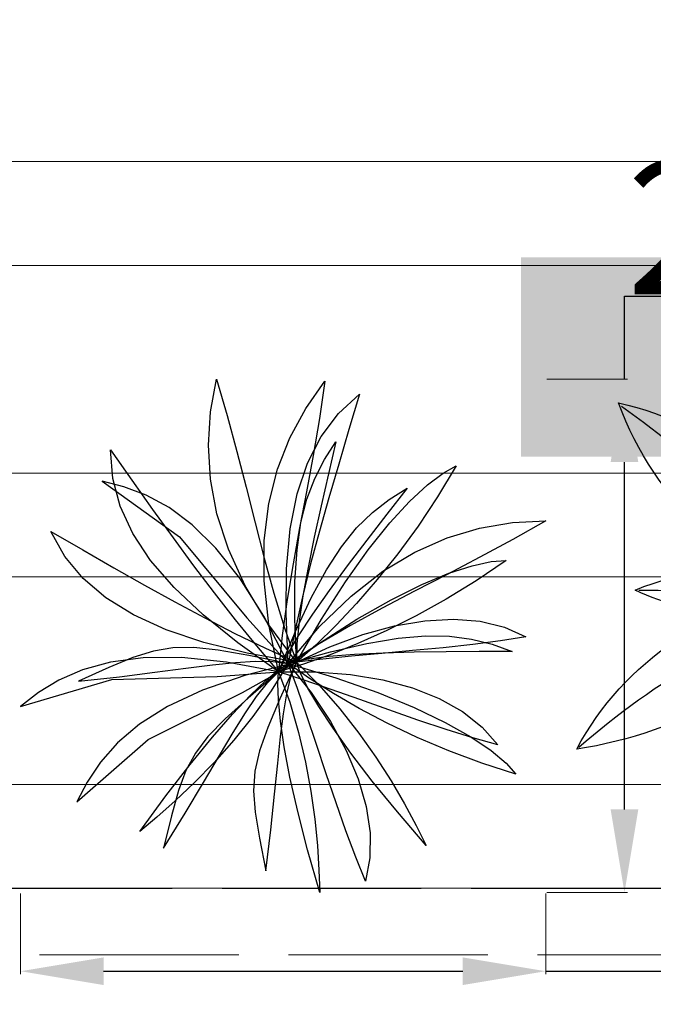
# Model space of a CAD drawing. Units: inches. Extents: x 351 to 1738, y -265 to 286.
# Tile 10 of 38: x 1074 to 1112, y -206 to -147. Entities that reach past the tile are written whole.
import ezdxf

# ---------------------------------------------------------------- set-up
doc = ezdxf.new("R2010")
doc.units = ezdxf.units.IN
doc.header["$MEASUREMENT"] = 0
doc.linetypes.add('ACAD_ISO02W100', pattern=[15, 12, -3])
for name, color, linetype, lineweight in [('A-ANNO-DIMS', 2, 'Continuous', 18), ('A-COLS-PATT', 6, 'Continuous', 13), ('A-FLOR-OVHD', 1, 'ACAD_ISO02W100', 18), ('A-FLOR-PATT', 9, 'Continuous', 9)]:
    doc.layers.add(name, color=color, linetype=linetype, lineweight=lineweight)
for name, color, linetype in [('CAY', 94, 'Continuous'), ('CHITIET', 144, 'Continuous'), ('DIENHOA', 3, 'Continuous'), ('netmanh', 9, 'Continuous'), ('VATDUNG', 9, 'Continuous')]:
    doc.layers.add(name, color=color, linetype=linetype)
doc.styles.get("Standard").update_dxf_attribs({"font": 'arial.ttf'})
doc.dimstyles.get("Standard").update_dxf_attribs({"dimtxt": 8, "dimasz": 5, "dimexe": 0.18, "dimexo": 0.0625, "dimgap": 0.09, "dimtad": 1, "dimtoh": 1, "dimzin": 0, "dimdsep": 46, "dimlunit": 4, "dimtxsty": 'Standard', "dimcen": 0, "dimclre": 256, "dimadec": 0, "dimazin": 0, "dimtfac": 1, "dimtofl": 0, "dimtmove": 0, "dimatfit": 3, "dimfxl": 1, "dimtolj": 1, "dimtzin": 0, "dimlwe": -1, "dimarcsym": 0})

# ---------------------------------------------------------------- blocks, each defined once
blk = doc.blocks.new('Cay03_mb')
at = {"layer": 'DIENHOA'}
for p, q in [((118.6, 555.3), (166.2, 599.1)), ((166.2, 599.1), (142.2, 519.4)), ((79.5, 503.7), (118.6, 555.3)), ((142.2, 519.4), (119, 441.7)), ((48.6, 443.6), (79.5, 503.7)), ((25.5, 374.3), (48.6, 443.6)), ((119, 441.7), (96.7, 365.6)), ((-365.2, 390.3), (-414.4, 402.8)), ((-414.4, 402.8), (-240.2, 277.8)), ((-314.9, 371.3), (-365.2, 390.3)), ((-263.5, 343.5), (-314.9, 371.3)), ((9.9, 295.3), (25.5, 374.3)), ((96.7, 365.6), (75.6, 290.6)), ((-211.2, 304.6), (-263.5, 343.5)), ((511, 309.6), (585.9, 313.5)), ((585.9, 313.5), (511.8, 271.4)), ((-158, 252.3), (-211.2, 304.6)), ((1.6, 205.7), (9.9, 295.3)), ((75.6, 290.6), (55.7, 216.3)), ((363.4, 275.4), (436.8, 297.2)), ((436.8, 297.2), (511, 309.6)), ((-240.2, 277.8), (-88.4, 94.9)), ((290.6, 243.2), (363.4, 275.4)), ((511.8, 271.4), (437.6, 231.5)), ((-104.2, 184.4), (-158, 252.3)), ((218.5, 199.8), (290.6, 243.2)), ((437.6, 231.5), (363.7, 192.9)), ((0.2, 104.9), (1.6, 205.7)), ((55.7, 216.3), (37.3, 142.1)), ((-49.6, 98.5), (-104.2, 184.4)), ((147, 144.1), (218.5, 199.8)), ((363.7, 192.9), (290.2, 154.9)), ((37.3, 142.1), (20.5, 67.6)), ((75.9, 75.2), (147, 144.1)), ((290.2, 154.9), (217.4, 116.6)), ((217.4, 116.6), (145.5, 77.3)), ((-88.4, 94.9), (5.4, -7.8)), ((5.4, -7.8), (-49.6, 98.5)), ((5.4, -7.8), (0.2, 104.9)), ((5.4, -7.8), (75.9, 75.2)), ((20.5, 67.6), (5.4, -7.8)), ((145.5, 77.3), (74.7, 36.1)), ((182.2, 37.2), (253, 48.9)), ((253, 48.9), (314.6, 54.1)), ((314.6, 54.1), (369.2, 53.3)), ((369.2, 53.3), (418.6, 46.8)), ((418.6, 46.8), (464.9, 35.2)), ((-254.7, 27.4), (-298.6, 20.1)), ((-208, 27.8), (-254.7, 27.4)), ((-152.7, 21.7), (-208, 27.8)), ((74.7, 36.1), (5.4, -7.8)), ((100.3, 18.4), (182.2, 37.2)), ((464.9, 35.2), (510, 19)), ((-345, 5.4), (-399.6, -17.1)), ((-298.6, 20.1), (-345, 5.4)), ((-83.4, 9.7), (-152.7, 21.7)), ((5.4, -7.8), (-83.4, 9.7)), ((5.4, -7.8), (100.3, 18.4)), ((46.3, 0.9), (5.4, -7.8)), ((96.7, 7.5), (46.3, 0.9)), ((155, 12.2), (96.7, 7.5)), ((219.6, 15.4), (155, 12.2)), ((289, 17.4), (219.6, 15.4)), ((361.6, 18.5), (289, 17.4)), ((435.8, 18.9), (361.6, 18.5)), ((510, 19), (435.8, 18.9)), ((-399.6, -17.1), (-468, -47.9)), ((-295.3, -27.9), (-225.8, -18.9)), ((-225.8, -18.9), (-165.8, -11.3)), ((-165.8, -11.3), (-114, -5.7)), ((-114, -5.7), (-69, -2.9)), ((-69, -2.9), (-29.6, -3.4)), ((5.4, -7.8), (-33.2, -69.5)), ((-29.6, -3.4), (5.4, -7.8)), ((-16.5, -22.4), (5.4, -7.8)), ((5.4, -7.8), (56.8, -73.3)), ((25.9, -64.4), (5.4, -7.8)), ((5.4, -7.8), (112.8, -40.3)), ((53.5, -41.6), (5.4, -7.8)), ((-468, -47.9), (-375.6, -37.8)), ((-375.6, -37.8), (-295.3, -27.9)), ((-45.1, -46.3), (-16.5, -22.4)), ((107, -75.7), (53.5, -41.6)), ((112.8, -40.3), (207.5, -73.8)), ((-79.8, -79.6), (-45.1, -46.3)), ((47, -125.9), (25.9, -64.4)), ((-120.2, -122.1), (-79.8, -79.6)), ((-33.2, -69.5), (-74.6, -127.3)), ((56.8, -73.3), (100.4, -139.1)), ((165.5, -109.6), (107, -75.7)), ((207.5, -73.8), (289.5, -107.6)), ((228.7, -142.8), (165.5, -109.6)), ((289.5, -107.6), (359.3, -141.1)), ((-165.9, -174.1), (-120.2, -122.1)), ((-74.6, -127.3), (-117.8, -181.1)), ((68.7, -190.6), (47, -125.9)), ((100.4, -139.1), (135.9, -204.3)), ((296, -174.7), (228.7, -142.8)), ((359.3, -141.1), (416.9, -173.5)), ((-216.3, -235.6), (-165.9, -174.1)), ((367.1, -204.8), (296, -174.7)), ((416.9, -173.5), (462.6, -204.2)), ((-117.8, -181.1), (-162.1, -230.9)), ((90.8, -256.6), (68.7, -190.6)), ((135.9, -204.3), (162.8, -268.3)), ((441.6, -232.7), (367.1, -204.8)), ((462.6, -204.2), (496.5, -232.5)), ((-271, -306.6), (-216.3, -235.6)), ((-162.1, -230.9), (-206.3, -276.5)), ((518.9, -257.7), (441.6, -232.7)), ((496.5, -232.5), (518.9, -257.7)), ((113.1, -322.2), (90.8, -256.6)), ((-206.3, -276.5), (-249.6, -317.8)), ((162.8, -268.3), (181, -330.4)), ((-329.5, -387.1), (-271, -306.6)), ((-249.6, -317.8), (-291, -354.7)), ((135.4, -385.6), (113.1, -322.2)), ((181, -330.4), (190, -390)), ((-291, -354.7), (-329.5, -387.1)), ((157.6, -445), (135.4, -385.6)), ((190, -390), (189.6, -446.3)), ((179.5, -498.7), (157.6, -445)), ((189.6, -446.3), (179.5, -498.7))]:
    blk.add_line(p, q, dxfattribs=at)
for points in [[(23.7, -5.4), (-41, 82.2), (-91.8, 167.1), (-129.7, 249.5), (-155.6, 329.6), (-170.2, 407.8), (-174.7, 484.2), (-169.8, 559.3), (-156.5, 633.1)], [(-156.5, 633.1), (-132.5, 551.3), (-110.5, 470), (-89.8, 389.2), (-69.6, 309), (-49, 229.4), (-27.1, 150.4), (-3.2, 72.1), (23.7, -5.4)], [(-16.4, -26.7), (-38.3, 80), (-48.9, 178.3), (-48.7, 269), (-38.5, 352.6), (-19.1, 429.7), (9, 501), (44.9, 567.1), (87.9, 628.5)], [(87.9, 628.5), (75.5, 544.2), (61.3, 461.2), (46.1, 379.1), (30.8, 297.8), (16.1, 216.9), (2.9, 136), (-8.3, 54.9), (-16.4, -26.7)], [(23.7, -5.4), (19.8, 93), (20.3, 177), (25, 248.5), (34, 309.8), (47.3, 362.7), (64.9, 409.3), (86.8, 451.7), (112.9, 491.9)], [(112.9, 491.9), (96, 419.7), (79.5, 347.4), (63.9, 276.5), (50, 208.4), (38.4, 144.8), (29.7, 86.9), (24.6, 36.3), (23.7, -5.4)], [(-395.6, 473.7), (-347.5, 405.6), (-300.6, 339.5), (-254.3, 275.1), (-208.3, 212.3), (-161.9, 150.9), (-114.8, 90.7), (-66.5, 31.6), (-16.4, -26.7)], [(-16.4, -26.7), (-108.3, 38.6), (-186.9, 101.7), (-252.4, 163.5), (-305.1, 224.4), (-345.4, 285.2), (-373.7, 346.6), (-390.4, 409.2), (-395.6, 473.7)], [(384.3, 437.5), (342.2, 367.8), (298.1, 301.7), (252.6, 239.4), (206.1, 181.1), (159.4, 127.2), (113, 78), (67.6, 33.6), (23.7, -5.4)], [(23.7, -5.4), (79.9, 91.7), (134.1, 176.2), (185.8, 248.4), (234.3, 308.7), (279, 357.3), (319.3, 394.8), (354.6, 421.4), (384.3, 437.5)], [(273.2, 387.3), (227.6, 328.8), (182.3, 270.1), (138.4, 212.3), (97.2, 156.4), (60, 103.4), (27.8, 54.6), (1.9, 10.8), (-16.4, -26.7)], [(-16.4, -26.7), (21.4, 64.2), (57, 140.3), (91.4, 203.3), (125.2, 255.1), (159.5, 297.5), (195, 332.5), (232.7, 361.8), (273.2, 387.3)], [(-530.5, 289.7), (-458.3, 248.1), (-387.9, 207.8), (-318.9, 168.7), (-250.8, 131.1), (-182.9, 94.8), (-114.9, 59.9), (-46.2, 26.5), (23.7, -5.4)], [(23.7, -5.4), (-87.2, 15.2), (-185, 39.6), (-270.3, 68.2), (-343.7, 101.4), (-405.9, 139.7), (-457.3, 183.5), (-498.7, 233.4), (-530.5, 289.7)], [(496.7, 224), (429.4, 178.4), (361.6, 136.9), (294.1, 99.5), (227.5, 66.1), (162.4, 36.7), (99.7, 11.5), (39.8, -9.7), (-16.4, -26.7)], [(-16.4, -26.7), (75.4, 37.9), (160.1, 91.8), (237.3, 135.7), (306.6, 170), (367.6, 195.4), (419.9, 212.5), (463.1, 221.9), (496.7, 224)], [(23.7, -5.4), (99.3, 29.7), (173.2, 57.1), (244.8, 76.7), (313.3, 88.3), (377.9, 91.8), (437.9, 87), (492.7, 73.8), (541.4, 52)], [(541.4, 52), (484.1, 42.9), (421.2, 34.8), (354.4, 27.6), (285.4, 20.9), (216.1, 14.5), (148.2, 8.1), (83.5, 1.6), (23.7, -5.4)], [(-16.4, -26.7), (-134, -4.7), (-235.3, 5.3), (-322, 4.7), (-395.9, -5), (-458.7, -22.3), (-512.3, -45.7), (-558.2, -73.6), (-598.4, -104.7)], [(-471.9, -320.3), (-310.5, -179.3), (-97.7, -73.3), (23.7, -5.4)], [(23.7, -5.4), (-92.3, -34.8), (-188.4, -68.2), (-266.9, -105.1), (-329.9, -144.9), (-379.7, -187), (-418.5, -230.7), (-448.5, -275.3), (-471.9, -320.3)], [(23.7, -5.4), (-13.6, -87.9), (-41.1, -152.6), (-59.6, -205), (-69.9, -250.7), (-72.8, -295), (-69.2, -343.6), (-59.7, -401.9), (-45.3, -475.5)], [(-45.3, -475.5), (-34.1, -383.2), (-25.4, -302.8), (-18.3, -233.1), (-12, -172.9), (-5.6, -121.2), (2, -76.8), (11.4, -38.5), (23.7, -5.4)], [(316.5, -418.1), (251.4, -342.8), (194.8, -273.3), (146.5, -210.2), (106.3, -153.8), (74.1, -104.7), (49.7, -63.4), (32.9, -30.1), (23.7, -5.4)], [(23.7, -5.4), (74.9, -57.1), (121.8, -110.6), (164.3, -165), (202.7, -219.4), (237, -272.9), (267.3, -324.5), (293.7, -373.2), (316.5, -418.1)], [(-598.4, -104.7), (-392.7, -44.4), (-155, -37.4), (-16.4, -26.7)], [(-276.2, -424.4), (-227.3, -345.4), (-185.7, -276.1), (-150, -215.7), (-119.1, -163.8), (-91.5, -119.5), (-66, -82.3), (-41.4, -51.6), (-16.4, -26.7)], [(-16.4, -26.7), (-84.9, -86), (-137, -133.1), (-175.8, -173), (-204.3, -210), (-225.5, -249.1), (-242.5, -294.7), (-258.4, -351.6), (-276.2, -424.4)], [(76.2, -524.2), (48.8, -428.5), (26.6, -341.7), (9.2, -264.1), (-3.6, -196.1), (-12.3, -138), (-17.1, -90.2), (-18.3, -53), (-16.4, -26.7)], [(-16.4, -26.7), (66.9, -26.6), (145.6, -32.7), (218.8, -44.9), (285.8, -63.1), (345.9, -87.1), (398.4, -116.6), (442.6, -151.6), (477.6, -191.8)], [(477.6, -191.8), (421.8, -176), (361.3, -156.9), (297.6, -135.5), (232.2, -112.6), (166.6, -89.4), (102.3, -66.6), (40.8, -45.4), (-16.4, -26.7)], [(-16.4, -26.7), (8.5, -95.1), (28.5, -163.3), (44.3, -230.6), (56.3, -296.1), (65, -359), (70.9, -418.5), (74.5, -473.9), (76.2, -524.2)]]:
    blk.add_lwpolyline(points, dxfattribs=at)
blk = doc.blocks.new('A$C5431134F')
at = {"layer": 'VATDUNG'}
for centre, radius, start, end in [((2160.8, 1662), 1245, 150.2411, 205.809), ((5177, 1582.5), 4150.3, 170.24, 186.1148), ((-65.9, 1738.8), 1267.2, 354.3326, 25.2804), ((1532.8, 1250.1), 499, 101.4267, 190.9877), ((193.1, 3473.3), 2507.8, 289.6318, 316.9416), ((2357.8, 162.2), 1629.1, 101.2486, 143.9899), ((1828.1, 1082.8), 773.2, 121.9055, 175.1859), ((1000.7, 2213.1), 1133.8, 274.4073, 336.4431), ((3715.1, 660.2), 2523.5, 154.6853, 162.4501), ((-246.7, 51.1), 1647.5, 39.15, 81.389), ((1000.7, 2213.1), 1133.8, 208.0484, 264.6491), ((1859.5, 3770.4), 2797.6, 228.5745, 252.3842), ((1101.5, 1552.5), 361.2, 169.1166, 218.9556), ((667.9, 1279.8), 349.9, 42.8374, 76.9786), ((-929.9, 388.9), 2082.1, 20.5138, 36.0242), ((1386.4, 1856.4), 738.5, 261.6389, 315.6255), ((-169.9, 6392.7), 5465.7, 286.3355, 292.415), ((1571.2, 1428.8), 356.3, 257.3557, 344.3532), ((624.5, 223.6), 940.4, 92.4374, 115.2956), ((-65.9, 1738.8), 1267.2, 330.7697, 331.9367), ((1294.4, -49.6), 1206.1, 104.1284, 160.1468), ((-2233.8, 3749.8), 4146.2, 305.4464, 320.7382), ((248.9, 8461.8), 7388, 269.91003, 274.50199), ((2052.7, 864.5), 1083.3, 166.3603, 232.9474), ((1250.8, 281.5), 836.9, 19.4342, 107.4357), ((625, 349.3), 851.8, 6.5073, 62.3609), ((754.1, -691.9), 1814.1, 46.1483, 80.3711), ((-70, 1420), 1084.7, 282.2423, 341.7321), ((546.4, 1826.6), 819.5, 246.7315, 287.3971), ((3885.3, 1488.7), 2894, 188.0959, 210.7226), ((1889.6, 1210.8), 871.9, 188.5552, 241.3289), ((-527.8, -458.7), 2192.5, 24.7599, 44.6473), ((2594.9, 3037.7), 2500, 231.5416, 257.1764), ((1738.9, 617.5), 897.6, 155.9893, 202.84), ((2946.5, 414), 2039.9, 165.0604, 184.0737), ((1214.1, 597.8), 452.1, 154.5276, 228.0163), ((-246.7, 51.1), 1647.5, 358.2222, 17.8583)]:
    blk.add_arc(centre, radius, start, end, dxfattribs=at)
blk = doc.blocks.new('A$C5A8625A6')
at = {"layer": 'CHITIET', "ltscale": 50, "xscale": -0.49, "yscale": 0.49, "zscale": 0.49, "rotation": 180}
blk.add_blockref('A$C5431134F', (0, 1120.2), dxfattribs=at)
blk = doc.blocks.new('A$C18571848')
at = {"layer": 'netmanh', "xscale": 0.5393606399999998, "yscale": 0.5393606399999998, "zscale": 0.5393606399999998}
blk.add_blockref('A$C5A8625A6', (0, 0), dxfattribs=at)
blk = doc.blocks.new('*D36')
at = {"layer": 'A-ANNO-DIMS', "transparency": 16777216}
for p, q in [((1073.569, -199.341), (1073.569, -204.202)), ((1105.198, -199.341), (1105.198, -204.202))]:
    blk.add_line(p, q, dxfattribs=at)
at = {"layer": 'A-ANNO-DIMS', "color": 0, "lineweight": -2, "transparency": 16777216}
for p, q in [((1078.569, -204.022), (1100.198, -204.022)), ((1105.198, -204.022), (1227.071, -204.022))]:
    blk.add_line(p, q, dxfattribs=at)
at = {"layer": 'A-ANNO-DIMS', "color": 0, "transparency": 16777216}
for points in [[(1078.569, -203.189), (1078.569, -204.856), (1073.569, -204.022)], [(1100.198, -203.189), (1100.198, -204.856), (1105.198, -204.022)]]:
    blk.add_solid(points, dxfattribs=at)
at = {"layer": 'Defpoints', "color": 0, "transparency": 16777216}
for p in [(1073.569, -199.278), (1105.198, -199.278), (1105.198, -204.022)]:
    blk.add_point(p, dxfattribs=at)
at = {"layer": 'A-ANNO-DIMS', "color": 0, "transparency": 16777216, "insert": (1168.634, -199.796), "char_height": 8, "attachment_point": 5}
blk.add_mtext('\\A1;PLANT A 2\'-7 1/2" TYP.', dxfattribs=at)
blk = doc.blocks.new('*D37')
at = {"layer": 'A-ANNO-DIMS', "color": 0, "lineweight": -2, "transparency": 16777216}
for p, q in [((1109.942, -168.369), (1109.942, -163.369)), ((1109.942, -163.369), (1158.933, -163.369)), ((1109.942, -194.278), (1109.942, -173.369))]:
    blk.add_line(p, q, dxfattribs=at)
at = {"layer": 'A-ANNO-DIMS', "transparency": 16777216}
for p, q in [((1105.26, -168.369), (1110.122, -168.369)), ((1105.26, -199.278), (1110.122, -199.278))]:
    blk.add_line(p, q, dxfattribs=at)
at = {"layer": 'A-ANNO-DIMS', "color": 0, "transparency": 16777216}
for points in [[(1109.109, -173.369), (1110.775, -173.369), (1109.942, -168.369)], [(1109.109, -194.278), (1110.775, -194.278), (1109.942, -199.278)]]:
    blk.add_solid(points, dxfattribs=at)
at = {"layer": 'Defpoints', "color": 0, "transparency": 16777216}
for p in [(1105.198, -168.369), (1109.942, -168.369), (1105.198, -199.278)]:
    blk.add_point(p, dxfattribs=at)
at = {"layer": 'A-ANNO-DIMS', "color": 0, "transparency": 16777216, "insert": (1134.482, -159.26), "char_height": 8, "attachment_point": 5}
blk.add_mtext('\\A1;2\'-7" TYP.', dxfattribs=at)

msp = doc.modelspace()

# ---------------------------------------------------------------- hatches: boundary and pattern name
at = {"layer": 'A-COLS-PATT'}
h = msp.add_hatch(color=256, dxfattribs=at)
h.dxf.hatch_style = 1
h.paths.add_polyline_path([(1112.704, 237.963), (1103.704, 237.963), (1103.704, 228.963), (1112.704, 228.963)])
h.paths.add_polyline_path([(1115.704, 237.963), (1112.704, 237.963), (1112.704, 228.963), (1115.704, 228.963)])
h.paths.add_polyline_path([(1043.704, 255.963), (1034.704, 255.963), (1034.704, 243.963), (1043.704, 243.963)])
h.paths.add_polyline_path([(1043.704, 210.963), (1034.704, 210.963), (1034.704, 198.963), (1043.704, 198.963)])
h.paths.add_polyline_path([(1043.704, -45.037), (1034.704, -45.037), (1034.704, -57.037), (1043.704, -57.037)])
h.paths.add_polyline_path([(1112.704, -45.037), (1103.704, -45.037), (1103.704, -57.037), (1112.704, -57.037)])
h.paths.add_polyline_path([(1112.704, -161.037), (1103.704, -161.037), (1103.704, -164.037), (1103.704, -173.037), (1112.704, -173.037)])
h.paths.add_polyline_path([(1043.704, -161.037), (1034.704, -161.037), (1034.704, -173.037), (1043.704, -173.037)])
h.paths.add_polyline_path([(1248.549, -164.037), (1236.549, -164.037), (1236.549, -173.037), (1248.549, -173.037)])
h.paths.add_polyline_path([(1248.549, -50), (1236.549, -50), (1236.549, -59), (1248.549, -59)])
h.paths.add_polyline_path([(1248.704, 73.463), (1244.704, 73.463), (1244.704, 64.463), (1248.704, 64.463)])
h.paths.add_polyline_path([(1244.704, 73.463), (1236.704, 73.463), (1236.704, 64.463), (1244.704, 64.463)])
h.paths.add_polyline_path([(1248.704, 237.963), (1236.704, 237.963), (1236.704, 228.963), (1248.704, 228.963)])
h.paths.add_polyline_path([(1392.204, 237.963), (1380.204, 237.963), (1380.204, 228.963), (1392.204, 228.963)])
h.paths.add_polyline_path([(1536.064, 237.963), (1524.064, 237.963), (1524.064, 228.963), (1536.064, 228.963)])
h.paths.add_polyline_path([(1536.064, 73.463), (1524.064, 73.463), (1524.064, 64.463), (1536.064, 64.463)])
h.paths.add_polyline_path([(1384.204, 73.463), (1380.204, 73.463), (1380.204, 64.463), (1384.204, 64.463)])
h.paths.add_polyline_path([(1392.064, 73.463), (1384.204, 73.463), (1384.204, 64.463), (1392.064, 64.463)])
h.paths.add_polyline_path([(1536.064, -53.037), (1524.064, -53.037), (1524.064, -57.037), (1536.064, -57.037)])
h.paths.add_polyline_path([(1536.064, -48.037), (1524.064, -48.037), (1524.064, -53.037), (1536.064, -53.037)])
h.paths.add_polyline_path([(1392.064, -48.037), (1380.064, -48.037), (1380.064, -56.5), (1380.065, -57.037), (1392.064, -57.037)])
h.paths.add_polyline_path([(1536.064, -164.037), (1524.064, -164.037), (1524.064, -173.037), (1536.064, -173.037)])
at = {"layer": 'A-FLOR-PATT', "transparency": 33554559}
h = msp.add_hatch(dxfattribs=at)
h.set_pattern_fill('ANSI32', color=256, scale=50, angle=135)
h.set_pattern_definition([(180, (1038.704, -199.037), (-2e-15, -18.75), []), (180, (1032.454, -192.787), (-2e-15, -18.75), [])])
h.paths.add_polyline_path([(1248.506, -102.915), (1236.559, -102.916), (1236.553, -56.864), (1112.704, -57.026), (1112.704, -57.037), (1103.704, -57.037), (1103.704, -45.037), (1103.704, 98.963), (1076.434, 98.963), (1076.549, -81.037), (1071.549, -81.037), (1043.704, -81.037), (1038.704, -81.037), (1038.704, -161.037), (1043.704, -161.037), (1043.704, -173.037), (1038.704, -173.037), (1038.704, -199.037), (1562.704, -199.037), (1562.704, -173.037), (1236.549, -173.037), (1236.549, -164.037), (1236.693, -164.037), (1236.676, -150.916), (1248.512, -150.915)])
h.paths.add_polyline_path([(1236.133, -134.078), (1247.348, -134.078), (1247.348, -122.929), (1236.133, -122.929)], flags=24)
h.paths.add_polyline_path([(1308.144, -185.548), (1321.66, -185.548), (1321.66, -174.4), (1308.144, -174.4)], flags=24)
h.paths.add_polyline_path([(1121.632, -122.88), (1179.647, -122.88), (1179.647, -112.309), (1121.632, -112.309)], flags=24)
h.paths.add_polyline_path([(1124.515, -112.593), (1177.986, -112.593), (1177.986, -101.056), (1124.515, -101.056)], flags=24)
h.paths.add_polyline_path([(1091.374, 23.58), (1104.89, 23.58), (1104.89, 34.728), (1091.374, 34.728)], flags=24)

# ---------------------------------------------------------------- linework, layer by layer
at = {"layer": 'A-FLOR-OVHD'}
for p, q in [((1562.704, -199.037), (1038.704, -199.037)), ((1566.704, -203.037), (1034.704, -203.037))]:
    msp.add_line(p, q, dxfattribs=at)

# ---------------------------------------------------------------- block references
at = {"layer": 'CAY'}
for name, p, xscale, yscale, zscale in [('A$C18571848', (1107.065, -200.223), 0.0597507335965459, 0.0597507335965459, 0.0597507335965459), ('Cay03_mb', (1089.549, -185.278), 0.0267074520028285, 0.0267074520028285, 0.0267074520028285)]:
    msp.add_blockref(name, p, dxfattribs=dict(at, xscale=xscale, yscale=yscale, zscale=zscale))

# ---------------------------------------------------------------- dimensions: what is measured, and where the dimension line sits
at = {"layer": 'A-ANNO-DIMS'}
dim = msp.add_linear_dim(base=(1109.942, -168.369), p1=(1105.198, -199.278), p2=(1105.198, -168.369), angle=90, text='<> TYP.', dimstyle='Standard', override={"dimdec": 1, "dimlfac": 1, "dimrnd": 0, "dimzin": 1, "dimdsep": 46, "dimlunit": 4, "dimfrac": 2}, dxfattribs=at)
dim.commit()
dim.dimension.update_dxf_attribs({"geometry": '*D37', "text_midpoint": (1134.482, -159.26)})
dim = msp.add_linear_dim(base=(1105.198, -204.022), p1=(1073.569, -199.278), p2=(1105.198, -199.278), text='PLANT A <> TYP.', dimstyle='Standard', override={"dimdec": 1, "dimlfac": 1, "dimrnd": 0, "dimzin": 1, "dimdsep": 46, "dimlunit": 4, "dimfrac": 2}, dxfattribs=at)
dim.commit()
dim.dimension.update_dxf_attribs({"geometry": '*D36', "text_midpoint": (1168.634, -199.796)})

doc.saveas('drawing.dxf')
